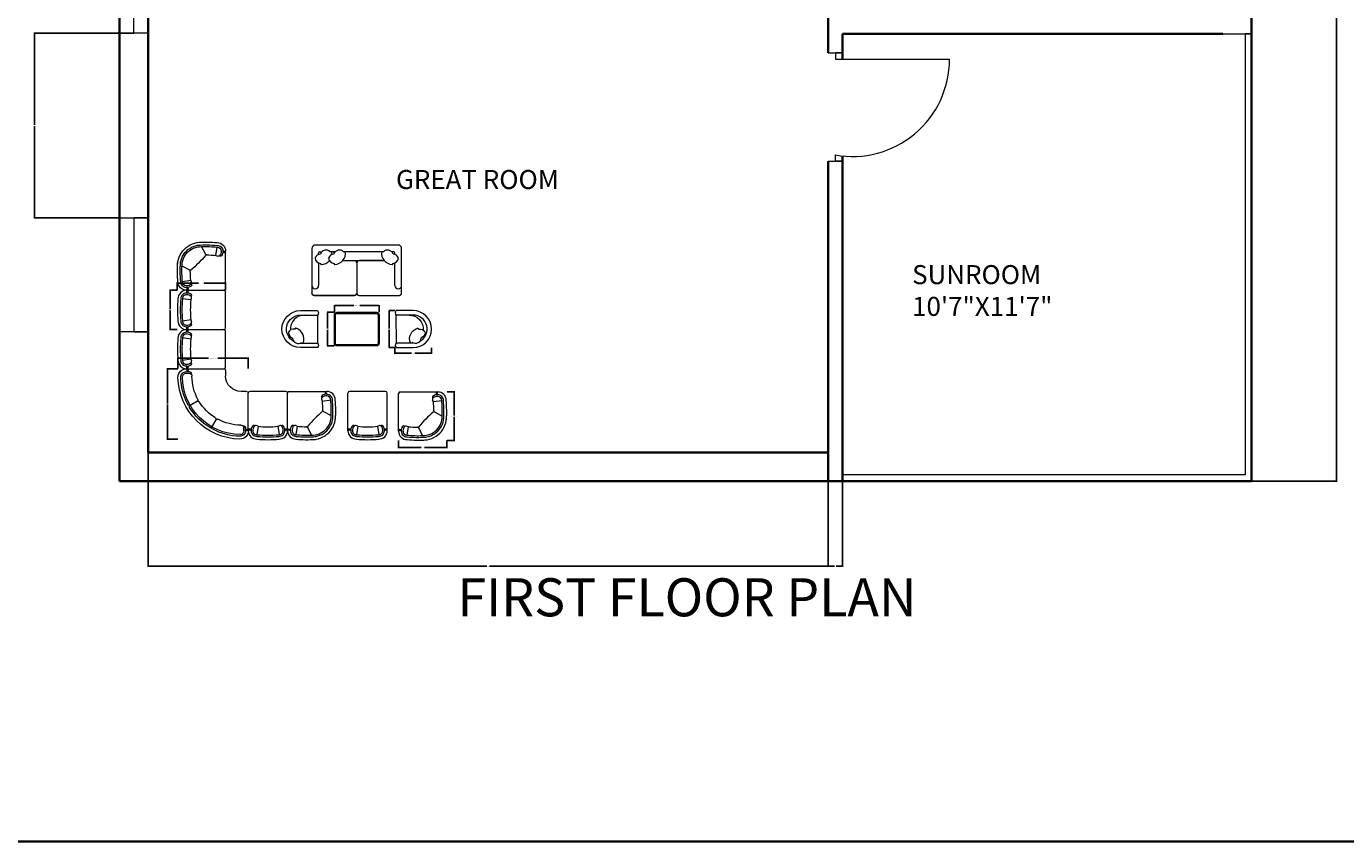
# Model space of a CAD drawing. Units: inches. Extents: x 1912 to 3731, y 1384 to 2459.
# Tile 3 of 8: x 2405 to 2821, y 1384 to 1641. Entities that reach past the tile are written whole.
import ezdxf

# ---------------------------------------------------------------- set-up
doc = ezdxf.new("R2010")
doc.units = ezdxf.units.IN
for name, color, linetype, lineweight in [('A-ANNO-DIMS', 2, 'Continuous', 18), ('A-ANNO-TITL', 7, 'Continuous', 25), ('A-ANNO-TTLB', 7, 'Continuous', 35), ('A-AREA-IDEN', 7, 'Continuous', 18), ('A-DOOR', 3, 'Continuous', 20), ('A-FURN', 8, 'Continuous', 15), ('A-GLAZ', 4, 'Continuous', 18), ('A-WALL', 7, 'Continuous', 35)]:
    doc.layers.add(name, color=color, linetype=linetype, lineweight=lineweight)
doc.styles.get("Standard").update_dxf_attribs({"font": 'arial.ttf'})
doc.dimstyles.get("Standard").update_dxf_attribs({"dimtxt": 0.18, "dimasz": 0.18, "dimexe": 0.18, "dimexo": 0.0625, "dimgap": 0.09, "dimtad": 0, "dimtih": 1, "dimtoh": 1, "dimdec": 4, "dimzin": 0, "dimdsep": 46, "dimtxsty": 'Standard', "dimcen": 0.09, "dimadec": 0, "dimazin": 0, "dimtfac": 1, "dimtdec": 4, "dimtofl": 0, "dimtmove": 0, "dimatfit": 3, "dimfxl": 1, "dimtolj": 1, "dimtzin": 0, "dimarcsym": 0})

# ---------------------------------------------------------------- blocks, each defined once
blk = doc.blocks.new('A$C707258B2')
at = {"color": 0}
for p, q in [((0.404, 0.342), (1.074, 0.342)), ((0.404, 0.292), (0.454, 0.292)), ((0.404, 0.262), (0.454, 0.262)), ((1.104, 0.312), (1.104, 0.212)), ((1.479, -0.063), (1.379, -0.063)), ((1.509, -0.763), (1.509, -0.093)), ((0.6, -0.238), (0.47, -0.313)), ((0.929, -0.567), (0.854, -0.697)), ((1.429, -0.763), (1.429, -0.713)), ((1.459, -0.763), (1.459, -0.712))]:
    blk.add_line(p, q, dxfattribs=at)
for centre, radius, start, end in [((0.404, 0.192), 0.15, 90, 181.1754), ((0.404, 0.192), 0.1, 90, 181.1754), ((0.404, 0.192), 0.07, 90, 181.1754), ((0.378, 0.317), 0.0362, 316.3972, 43.6028), ((0.368, 0.317), 0.0662, 337.8298, 22.1702), ((0.455, 0.256), 0.0357, 345.4262, 90.5555), ((0.454, 0.212), 0.05, 360, 90), ((1.074, 0.312), 0.03, 360, 90), ((1.379, 0.212), 1.125, 181.1754, 268.8246), ((1.379, 0.212), 1.075, 181.1754, 208.6357), ((1.379, 0.212), 1.045, 181.1754, 268.8246), ((1.379, 0.212), 0.875, 180, 208.4082), ((1.379, 0.212), 0.275, 180, 270), ((0.587, -0.216), 0.025, 300, 28.4082), ((0.612, -0.259), 0.025, 31.5918, 120), ((1.479, -0.093), 0.03, 360, 90), ((0.457, -0.291), 0.025, 208.6357, 300), ((0.482, -0.334), 0.025, 120, 211.3643), ((1.379, 0.212), 1.075, 211.3643, 238.6357), ((1.379, 0.212), 0.875, 211.5918, 238.4082), ((0.832, -0.685), 0.025, 238.6357, 330), ((0.876, -0.71), 0.025, 150, 241.3643), ((0.907, -0.555), 0.025, 330, 58.4082), ((0.951, -0.58), 0.025, 61.5918, 150), ((1.379, 0.212), 0.875, 241.5918, 270), ((1.379, -0.713), 0.05, 360, 90), ((1.425, -0.709), 0.0336, 354.6301, 109.3883), ((1.379, 0.212), 1.075, 241.3643, 268.8246), ((1.359, -0.763), 0.15, 268.8246, 360), ((1.359, -0.763), 0.1, 268.8246, 360), ((1.359, -0.763), 0.07, 268.8246, 360), ((1.484, -0.799), 0.0662, 67.8298, 112.1702), ((1.484, -0.789), 0.0362, 46.3972, 133.6028)]:
    blk.add_arc(centre, radius, start, end, dxfattribs=at)
blk = doc.blocks.new('A$C1352')
at = {"color": 0}
for points in [[(0.003, 0.053), (0.003, 0.553, -0.414214), (0.053, 0.603), (0.753, 0.603, -0.414214), (0.803, 0.553), (0.803, 0.053, -0.414214), (0.753, 0.003), (0.053, 0.003, -0.414214)], [(0.023, 0.053), (0.023, 0.553, -0.414214), (0.053, 0.583), (0.753, 0.583, -0.414214), (0.783, 0.553), (0.783, 0.053, -0.414214), (0.753, 0.023), (0.053, 0.023, -0.414214)]]:
    blk.add_lwpolyline(points, format="xyb", close=True, dxfattribs=at)
blk = doc.blocks.new('part 01')
at = {"color": 0}
for p, q in [((-591, 527), (-740, 550)), ((-670, 700), (0, 700)), ((-591, 527), (-579, 561)), ((30, 30), (30, 670)), ((-591, 173), (-740, 150)), ((-670, 0), (0, 0)), ((-591, 173), (-579, 139))]:
    blk.add_line(p, q, dxfattribs=at)
for centre, radius, start, end in [((1178, 350), 2008, 174.2835, 185.7165), ((-670, 550), 150, 90, 181.1754), ((1178, 350), 1958, 174.2835, 185.7165), ((-670, 550), 100, 90, 181.1754), ((1178, 350), 1928, 174.2835, 185.7165), ((-670, 550), 70, 90, 181.1754), ((-660, 518), 133, 56.0897, 95.6132), ((-696, 675), 36.2, 316.3972, 43.6028), ((-660, 518), 103, 42.0066, 95.6132), ((-706, 675), 66.2, 337.8298, 22.1702), ((1178, 350), 1778, 174.2835, 185.7165), ((-600, 607), 25, 332.9608, 56.0897), ((-625, 620), 53.2, 321.0017, 332.9608), ((-602, 570), 25, 340, 42.0066), ((0, 670), 30, 0, 90), ((-670, 150), 150, 178.8246, 270), ((-670, 150), 100, 178.8246, 270), ((-670, 150), 70, 178.8246, 270), ((-660, 182), 133, 264.3868, 303.9103), ((-660, 182), 103, 264.3868, 317.9934), ((-696, 25), 36.2, 316.3972, 43.6028), ((-706, 25), 66.2, 337.8298, 22.1702), ((-600, 93), 25, 303.9103, 27.0392), ((-602, 130), 25, 317.9934, 20), ((-625, 80), 53.2, 27.0392, 38.9983), ((0, 30), 30, 270, 0)]:
    blk.add_arc(centre, radius, start, end, dxfattribs=at)
blk = doc.blocks.new('part02')
at = {"color": 0}
for p, q in [((0, -670), (0, 0)), ((30, 30), (700, 30)), ((621, -143), (609, -109)), ((621, -143), (770, -120)), ((640, -326), (778, -399)), ((173, -591), (139, -579)), ((173, -591), (150, -740)), ((356, -610), (429, -748))]:
    blk.add_line(p, q, dxfattribs=at)
for centre, radius, start, end in [((30, 0), 30, 90, 180), ((726, 5), 56.2, 153.6122, 206.6666), ((726, 5), 36.2, 136.3972, 223.6028), ((700, -120), 150, 0, 90), ((630, -63), 25, 123.9103, 207.0392), ((655, -50), 53.2, 207.0392, 218.9983), ((632, -100), 25, 137.9934, 200), ((690, -152), 103, 84.3868, 137.9934), ((689, -151), 132, 85.4378, 123.9887), ((-1148, -320), 1778, 0.3836, 5.7165), ((700, -121), 101, 357.5006, 89.858), ((700, -120), 70, 0, 90), ((-1228, -320), 2008, 357.7349, 5.7032), ((-1148, -320), 1958, 355.8657, 5.7165), ((-1148, -320), 2008, 355.818, 5.7165), ((2220, -2190), 2454, 130.6961, 139.3039), ((439, -409), 419, 268.2181, 1.7819), ((439, -409), 369, 268.2181, 1.7819), ((439, -409), 339, 268.2181, 1.7819), ((632, -344), 20, 62, 130.6961), ((650, -308), 20, 180.3836, 242), ((25, -696), 56.2, 63.3334, 116.3878), ((25, -696), 36.2, 46.3972, 133.6028), ((150, -670), 150, 180, 271.1754), ((182, -660), 133, 146.0897, 185.6132), ((150, -670), 100, 180, 271.1754), ((93, -600), 25, 62.9608, 146.0897), ((182, -660), 103, 132.0066, 185.6132), ((150, -670), 70, 180, 270), ((80, -625), 53.2, 51.0017, 62.9608), ((130, -602), 25, 70, 132.0066), ((350, 1178), 1778, 264.2835, 269.6164), ((338, -620), 20, 28, 89.6164), ((374, -602), 20, 139.3039, 208), ((350, 1258), 2008, 264.2968, 272.2651), ((350, 1178), 2008, 264.2835, 274.182), ((350, 1178), 1958, 264.2835, 274.1343)]:
    blk.add_arc(centre, radius, start, end, dxfattribs=at)
blk = doc.blocks.new('LOUNGE-CHAIR')
blk.add_line((5.83, 1.42), (11.22, 1.41))
at = {"ltscale": 0.03}
blk.add_lwpolyline([(11.22, 1.41, -0.369229), (11.22, 0), (5.83, 0, -1), (5.84, 11.67), (11.23, 11.67, -0.369229), (11.23, 10.25)], format="xyb", close=True, dxfattribs=at)
blk.add_lwpolyline([(3.79, 1.92, -0.785087), (5.84, 10.26), (11.23, 10.25)], format="xyb")
for centre, radius, start, end in [((7.08, 5.84), 4.42, 89.9461, 183.658), ((3.71, 4.07), 1.82, 76.6403, 159.4695), ((4, 4.88), 1.99, 184.9999, 251.3534), ((4.33, 5.92), 0.211, 60.6238, 203.7423), ((3.5, 2.81), 3.42, 337.0143, 74.2857), ((5.13, 3.08), 1.77, 182.9922, 304.1401), ((5.83, 5.84), 4.42, 268.8536, 269.9461)]:
    blk.add_arc(centre, radius, start, end)
blk = doc.blocks.new('DOOR-36-FF-SUNROOM')
for p, q in [((0, 34.16), (4.5, 34.16)), ((4.5, 34.16), (2.25, 34.16)), ((2.25, 34.16), (2.25, 32.16)), ((2.25, 32.16), (38.25, 32.16)), ((2.25, 0), (2.25, 2)), ((0, 0), (4.5, 0)), ((4.5, 0), (2.25, 0))]:
    blk.add_line(p, q)
blk.add_arc((7.62, 32.16), 30.63, 259.9112, 0)
blk = doc.blocks.new('WIN-PLAN-60-B')
for p, q in [((0, 60), (9, 60)), ((9, 60), (4.5, 60)), ((4.5, 60), (4.5, 0)), ((9, 0), (0, 0)), ((4.5, 0), (9, 0))]:
    blk.add_line(p, q)
blk = doc.blocks.new('WIN-PLAN-36')
for p, q in [((4.5, 36), (0, 36)), ((0, 36), (9, 36)), ((4.5, 0), (4.5, 36)), ((9, 0), (0, 0)), ((0, 0), (4.5, 0))]:
    blk.add_line(p, q)
blk = doc.blocks.new('*D51')
at = {"layer": 'A-ANNO-DIMS', "color": 0, "lineweight": -2, "transparency": 16777216}
for p, q in [((2521.09, 1551.36), (2519.22, 1551.36)), ((2519.4, 1551.18), (2519.4, 1545.7)), ((2519.4, 1539.86), (2519.4, 1545.34)), ((2521.09, 1539.68), (2519.22, 1539.68))]:
    blk.add_line(p, q, dxfattribs=at)
at = {"layer": 'A-ANNO-DIMS', "color": 0, "transparency": 16777216}
for points in [[(2519.37, 1551.18), (2519.43, 1551.18), (2519.4, 1551.36)], [(2519.37, 1539.86), (2519.43, 1539.86), (2519.4, 1539.68)]]:
    blk.add_solid(points, dxfattribs=at)
at = {"layer": 'Defpoints', "color": 0, "transparency": 16777216}
for p in [(2519.4, 1551.36), (2521.15, 1551.36), (2521.15, 1539.68)]:
    blk.add_point(p, dxfattribs=at)
at = {"layer": 'A-ANNO-DIMS', "color": 0, "transparency": 16777216, "insert": (2519.4, 1545.52), "char_height": 0.18, "attachment_point": 5}
blk.add_mtext('\\A1;CHAIR 12 TYP.', dxfattribs=at)
blk = doc.blocks.new('*D52')
at = {"layer": 'A-ANNO-DIMS', "color": 0, "lineweight": -2, "transparency": 16777216}
for p, q in [((2521.15, 1539.62), (2521.15, 1537.75)), ((2532.73, 1539.62), (2532.73, 1537.75)), ((2521.33, 1537.93), (2526.42, 1537.93)), ((2532.55, 1537.93), (2527.46, 1537.93))]:
    blk.add_line(p, q, dxfattribs=at)
at = {"layer": 'A-ANNO-DIMS', "color": 0, "transparency": 16777216}
for points in [[(2521.33, 1537.96), (2521.33, 1537.9), (2521.15, 1537.93)], [(2532.55, 1537.96), (2532.55, 1537.9), (2532.73, 1537.93)]]:
    blk.add_solid(points, dxfattribs=at)
at = {"layer": 'Defpoints', "color": 0, "transparency": 16777216}
for p in [(2521.15, 1539.68), (2532.73, 1539.68), (2521.15, 1537.93)]:
    blk.add_point(p, dxfattribs=at)
at = {"layer": 'A-ANNO-DIMS', "color": 0, "transparency": 16777216, "insert": (2526.94, 1537.93), "char_height": 0.18, "attachment_point": 5}
blk.add_mtext('\\A1;12 TYP.', dxfattribs=at)
blk = doc.blocks.new('*D53')
at = {"layer": 'A-ANNO-DIMS', "color": 0, "lineweight": -2, "transparency": 16777216}
for p, q in [((2452.52, 1557.83), (2452.52, 1560.24)), ((2467.77, 1557.83), (2467.77, 1560.24)), ((2452.7, 1560.06), (2459.25, 1560.06)), ((2467.59, 1560.06), (2461.04, 1560.06))]:
    blk.add_line(p, q, dxfattribs=at)
at = {"layer": 'A-ANNO-DIMS', "color": 0, "transparency": 16777216}
for points in [[(2452.7, 1560.09), (2452.7, 1560.03), (2452.52, 1560.06)], [(2467.59, 1560.09), (2467.59, 1560.03), (2467.77, 1560.06)]]:
    blk.add_solid(points, dxfattribs=at)
at = {"layer": 'Defpoints', "color": 0, "transparency": 16777216}
for p in [(2452.52, 1557.77), (2467.77, 1560.06), (2467.77, 1557.77)]:
    blk.add_point(p, dxfattribs=at)
at = {"layer": 'A-ANNO-DIMS', "color": 0, "transparency": 16777216, "insert": (2460.15, 1560.06), "char_height": 0.18, "attachment_point": 5}
blk.add_mtext('\\A1;SEAT 15 TYP.', dxfattribs=at)
blk = doc.blocks.new('*D54')
at = {"layer": 'A-ANNO-DIMS', "color": 0, "lineweight": -2, "transparency": 16777216}
for p, q in [((2452.45, 1557.77), (2450.05, 1557.77)), ((2450.23, 1557.59), (2450.23, 1551.76)), ((2450.23, 1545.57), (2450.23, 1551.4)), ((2452.45, 1545.39), (2450.05, 1545.39))]:
    blk.add_line(p, q, dxfattribs=at)
at = {"layer": 'A-ANNO-DIMS', "color": 0, "transparency": 16777216}
for points in [[(2450.2, 1557.59), (2450.26, 1557.59), (2450.23, 1557.77)], [(2450.2, 1545.57), (2450.26, 1545.57), (2450.23, 1545.39)]]:
    blk.add_solid(points, dxfattribs=at)
at = {"layer": 'Defpoints', "color": 0, "transparency": 16777216}
for p in [(2450.23, 1557.77), (2452.52, 1557.77), (2452.52, 1545.39)]:
    blk.add_point(p, dxfattribs=at)
at = {"layer": 'A-ANNO-DIMS', "color": 0, "transparency": 16777216, "insert": (2450.23, 1551.58), "char_height": 0.18, "attachment_point": 5}
blk.add_mtext('\\A1;12 TYP.', dxfattribs=at)
blk = doc.blocks.new('*D55')
at = {"layer": 'A-ANNO-DIMS', "color": 0, "lineweight": -2, "transparency": 16777216}
for p, q in [((2537.62, 1525.71), (2540.02, 1525.71)), ((2539.84, 1525.53), (2539.84, 1518.27)), ((2539.84, 1510.64), (2539.84, 1517.91)), ((2537.62, 1510.46), (2540.02, 1510.46))]:
    blk.add_line(p, q, dxfattribs=at)
at = {"layer": 'A-ANNO-DIMS', "color": 0, "transparency": 16777216}
for points in [[(2539.81, 1525.53), (2539.87, 1525.53), (2539.84, 1525.71)], [(2539.81, 1510.64), (2539.87, 1510.64), (2539.84, 1510.46)]]:
    blk.add_solid(points, dxfattribs=at)
at = {"layer": 'Defpoints', "color": 0, "transparency": 16777216}
for p in [(2537.56, 1525.71), (2539.84, 1525.71), (2537.56, 1510.46)]:
    blk.add_point(p, dxfattribs=at)
at = {"layer": 'A-ANNO-DIMS', "color": 0, "transparency": 16777216, "insert": (2539.84, 1518.09), "char_height": 0.18, "attachment_point": 5}
blk.add_mtext('\\A1;END SEAT 15 TYP.', dxfattribs=at)
blk = doc.blocks.new('*D56')
at = {"layer": 'A-ANNO-DIMS', "color": 0, "lineweight": -2, "transparency": 16777216}
for p, q in [((2522.3, 1510.4), (2522.3, 1508)), ((2537.56, 1510.4), (2537.56, 1508)), ((2522.48, 1508.18), (2529.41, 1508.18)), ((2537.38, 1508.18), (2530.45, 1508.18))]:
    blk.add_line(p, q, dxfattribs=at)
at = {"layer": 'A-ANNO-DIMS', "color": 0, "transparency": 16777216}
for points in [[(2522.48, 1508.21), (2522.48, 1508.15), (2522.3, 1508.18)], [(2537.38, 1508.21), (2537.38, 1508.15), (2537.56, 1508.18)]]:
    blk.add_solid(points, dxfattribs=at)
at = {"layer": 'Defpoints', "color": 0, "transparency": 16777216}
for p in [(2522.3, 1510.46), (2537.56, 1510.46), (2537.56, 1508.18)]:
    blk.add_point(p, dxfattribs=at)
at = {"layer": 'A-ANNO-DIMS', "color": 0, "transparency": 16777216, "insert": (2529.93, 1508.18), "char_height": 0.18, "attachment_point": 5}
blk.add_mtext('\\A1;15 TYP.', dxfattribs=at)
blk = doc.blocks.new('*D57')
at = {"layer": 'A-ANNO-DIMS', "color": 0, "lineweight": -2, "transparency": 16777216}
for p, q in [((2452.74, 1533.08), (2452.74, 1536.53)), ((2452.92, 1536.35), (2462.36, 1536.35)), ((2474.75, 1536.35), (2465.31, 1536.35)), ((2474.93, 1533.08), (2474.93, 1536.53))]:
    blk.add_line(p, q, dxfattribs=at)
at = {"layer": 'A-ANNO-DIMS', "color": 0, "transparency": 16777216}
for points in [[(2452.92, 1536.38), (2452.92, 1536.32), (2452.74, 1536.35)], [(2474.75, 1536.38), (2474.75, 1536.32), (2474.93, 1536.35)]]:
    blk.add_solid(points, dxfattribs=at)
at = {"layer": 'Defpoints', "color": 0, "transparency": 16777216}
for p in [(2474.93, 1536.35), (2452.74, 1533.02), (2474.93, 1533.02)]:
    blk.add_point(p, dxfattribs=at)
at = {"layer": 'A-ANNO-DIMS', "color": 0, "transparency": 16777216, "insert": (2463.83, 1536.35), "char_height": 0.18, "attachment_point": 5}
blk.add_mtext('\\A1;CORNER SEAT 22 TYP.', dxfattribs=at)
blk = doc.blocks.new('*D58')
at = {"layer": 'A-ANNO-DIMS', "color": 0, "lineweight": -2, "transparency": 16777216}
for p, q in [((2452.68, 1533.02), (2449.23, 1533.02)), ((2449.41, 1532.84), (2449.41, 1522.11)), ((2449.41, 1511.01), (2449.41, 1521.74)), ((2452.68, 1510.83), (2449.23, 1510.83))]:
    blk.add_line(p, q, dxfattribs=at)
at = {"layer": 'A-ANNO-DIMS', "color": 0, "transparency": 16777216}
for points in [[(2449.38, 1532.84), (2449.44, 1532.84), (2449.41, 1533.02)], [(2449.38, 1511.01), (2449.44, 1511.01), (2449.41, 1510.83)]]:
    blk.add_solid(points, dxfattribs=at)
at = {"layer": 'Defpoints', "color": 0, "transparency": 16777216}
for p in [(2449.41, 1533.02), (2452.74, 1533.02), (2452.74, 1510.83)]:
    blk.add_point(p, dxfattribs=at)
at = {"layer": 'A-ANNO-DIMS', "color": 0, "transparency": 16777216, "insert": (2449.41, 1521.92), "char_height": 0.18, "attachment_point": 5}
blk.add_mtext('\\A1;22 TYP.', dxfattribs=at)
blk = doc.blocks.new('*D59')
at = {"layer": 'A-ANNO-DIMS', "color": 0, "lineweight": -2, "transparency": 16777216}
for p, q in [((2502.06, 1550.88), (2502.06, 1553.12)), ((2502.24, 1552.94), (2508.17, 1552.94)), ((2516.02, 1552.94), (2510.1, 1552.94)), ((2516.2, 1550.88), (2516.2, 1553.12))]:
    blk.add_line(p, q, dxfattribs=at)
at = {"layer": 'A-ANNO-DIMS', "color": 0, "transparency": 16777216}
for points in [[(2502.24, 1552.97), (2502.24, 1552.91), (2502.06, 1552.94)], [(2516.02, 1552.97), (2516.02, 1552.91), (2516.2, 1552.94)]]:
    blk.add_solid(points, dxfattribs=at)
at = {"layer": 'Defpoints', "color": 0, "transparency": 16777216}
for p in [(2516.2, 1552.94), (2502.06, 1550.82), (2516.2, 1550.82)]:
    blk.add_point(p, dxfattribs=at)
at = {"layer": 'A-ANNO-DIMS', "color": 0, "transparency": 16777216, "insert": (2509.13, 1552.94), "char_height": 0.18, "attachment_point": 5}
blk.add_mtext('\\A1;TABLE 14 TYP.', dxfattribs=at)
blk = doc.blocks.new('*D60')
at = {"layer": 'A-ANNO-DIMS', "color": 0, "lineweight": -2, "transparency": 16777216}
for p, q in [((2502, 1550.82), (2499.76, 1550.82)), ((2499.94, 1550.64), (2499.94, 1545.7)), ((2499.94, 1540.39), (2499.94, 1545.34)), ((2502, 1540.21), (2499.76, 1540.21))]:
    blk.add_line(p, q, dxfattribs=at)
at = {"layer": 'A-ANNO-DIMS', "color": 0, "transparency": 16777216}
for points in [[(2499.91, 1550.64), (2499.97, 1550.64), (2499.94, 1550.82)], [(2499.91, 1540.39), (2499.97, 1540.39), (2499.94, 1540.21)]]:
    blk.add_solid(points, dxfattribs=at)
at = {"layer": 'Defpoints', "color": 0, "transparency": 16777216}
for p in [(2499.94, 1550.82), (2502.06, 1550.82), (2502.06, 1540.21)]:
    blk.add_point(p, dxfattribs=at)
at = {"layer": 'A-ANNO-DIMS', "color": 0, "transparency": 16777216, "insert": (2499.94, 1545.52), "char_height": 0.18, "attachment_point": 5}
blk.add_mtext('\\A1;11 TYP.', dxfattribs=at)
blk = doc.blocks.new('*D100')
at = {"layer": 'A-ANNO-DIMS', "color": 0, "lineweight": -2, "transparency": 16777216}
for p, q in [((2791.37, 1973.13), (2818.34, 1973.13)), ((2818.16, 1972.95), (2818.16, 1735.56)), ((2818.16, 1497.81), (2818.16, 1735.19)), ((2791.37, 1497.63), (2818.34, 1497.63))]:
    blk.add_line(p, q, dxfattribs=at)
at = {"layer": 'A-ANNO-DIMS', "color": 0, "transparency": 16777216}
for points in [[(2818.13, 1972.95), (2818.19, 1972.95), (2818.16, 1973.13)], [(2818.13, 1497.81), (2818.19, 1497.81), (2818.16, 1497.63)]]:
    blk.add_solid(points, dxfattribs=at)
at = {"layer": 'Defpoints', "color": 0, "transparency": 16777216}
for p in [(2791.31, 1973.13), (2818.16, 1973.13), (2791.31, 1497.63)]:
    blk.add_point(p, dxfattribs=at)
at = {"layer": 'A-ANNO-DIMS', "color": 0, "transparency": 16777216, "insert": (2818.16, 1735.38), "char_height": 0.18, "attachment_point": 5}
blk.add_mtext('\\A1;475.5', dxfattribs=at)
blk = doc.blocks.new('*D102')
at = {"layer": 'A-ANNO-DIMS', "color": 0, "lineweight": -2, "transparency": 16777216}
for p, q in [((2434.25, 1638.78), (2407.28, 1638.78)), ((2407.46, 1638.6), (2407.46, 1609.89)), ((2407.46, 1580.82), (2407.46, 1609.53)), ((2434.25, 1580.64), (2407.28, 1580.64))]:
    blk.add_line(p, q, dxfattribs=at)
at = {"layer": 'A-ANNO-DIMS', "color": 0, "transparency": 16777216}
for points in [[(2407.43, 1638.6), (2407.49, 1638.6), (2407.46, 1638.78)], [(2407.43, 1580.82), (2407.49, 1580.82), (2407.46, 1580.64)]]:
    blk.add_solid(points, dxfattribs=at)
at = {"layer": 'Defpoints', "color": 0, "transparency": 16777216}
for p in [(2407.46, 1638.78), (2434.31, 1638.78), (2434.31, 1580.64)]:
    blk.add_point(p, dxfattribs=at)
at = {"layer": 'A-ANNO-DIMS', "color": 0, "transparency": 16777216, "insert": (2407.46, 1609.71), "char_height": 0.18, "attachment_point": 5}
blk.add_mtext('\\A1;58.15', dxfattribs=at)
blk = doc.blocks.new('*D103')
at = {"layer": 'A-ANNO-DIMS', "color": 0, "lineweight": -2, "transparency": 16777216}
for p, q in [((2443.31, 1506.56), (2443.31, 1470.6)), ((2657.81, 1506.56), (2657.81, 1470.6)), ((2443.49, 1470.78), (2550.17, 1470.78)), ((2657.63, 1470.78), (2550.96, 1470.78))]:
    blk.add_line(p, q, dxfattribs=at)
at = {"layer": 'A-ANNO-DIMS', "color": 0, "transparency": 16777216}
for points in [[(2443.49, 1470.81), (2443.49, 1470.75), (2443.31, 1470.78)], [(2657.63, 1470.81), (2657.63, 1470.75), (2657.81, 1470.78)]]:
    blk.add_solid(points, dxfattribs=at)
at = {"layer": 'Defpoints', "color": 0, "transparency": 16777216}
for p in [(2443.31, 1506.63), (2657.81, 1506.63), (2657.81, 1470.78)]:
    blk.add_point(p, dxfattribs=at)
at = {"layer": 'A-ANNO-DIMS', "color": 0, "transparency": 16777216, "insert": (2550.56, 1470.78), "char_height": 0.18, "attachment_point": 5}
blk.add_mtext('\\A1;214.5', dxfattribs=at)
blk = doc.blocks.new('*D104')
at = {"layer": 'A-ANNO-DIMS', "color": 0, "lineweight": -2, "transparency": 16777216}
for p, q in [((2657.81, 1497.56), (2657.81, 1470.6)), ((2662.31, 1497.56), (2662.31, 1470.6)), ((2657.99, 1470.78), (2659.8, 1470.78)), ((2662.13, 1470.78), (2660.32, 1470.78))]:
    blk.add_line(p, q, dxfattribs=at)
at = {"layer": 'A-ANNO-DIMS', "color": 0, "transparency": 16777216}
for points in [[(2657.99, 1470.81), (2657.99, 1470.75), (2657.81, 1470.78)], [(2662.13, 1470.81), (2662.13, 1470.75), (2662.31, 1470.78)]]:
    blk.add_solid(points, dxfattribs=at)
at = {"layer": 'Defpoints', "color": 0, "transparency": 16777216}
for p in [(2657.81, 1497.63), (2662.31, 1497.63), (2662.31, 1470.78)]:
    blk.add_point(p, dxfattribs=at)
at = {"layer": 'A-ANNO-DIMS', "color": 0, "transparency": 16777216, "insert": (2660.06, 1470.78), "char_height": 0.18, "attachment_point": 5}
blk.add_mtext('\\A1;4.5', dxfattribs=at)

msp = doc.modelspace()

# ---------------------------------------------------------------- linework, layer by layer
at = {"layer": 'A-ANNO-TTLB'}
msp.add_lwpolyline([(1912.2029, 2458.5537), (3720.218, 2458.5537), (3720.218, 1383.9599), (1912.2029, 1383.9599)], close=True, dxfattribs=at)
at = {"layer": 'A-FURN'}
for p, q in [((2497.1144, 1569.0629), (2497.1144, 1569.5551)), ((2497.4679, 1569.9086), (2498.1182, 1569.9086)), ((2502.3619, 1569.9086), (2500.6702, 1569.9086)), ((2501.7116, 1569.9086), (2502.3619, 1569.9086)), ((2517.597, 1569.9086), (2504.9139, 1569.9086)), ((2520.7994, 1569.9086), (2520.149, 1569.9086)), ((2521.1529, 1569.0629), (2521.1529, 1569.5551)), ((2497.1144, 1566.3798), (2497.1144, 1559.3034)), ((2521.1529, 1559.3034), (2521.1529, 1566.3798))]:
    msp.add_line(p, q, dxfattribs=at)
at = {"layer": 'A-FURN', "ltscale": 0.03}
msp.add_lwpolyline([(2509.1423, 1556.8289, 0.41421356), (2509.8493, 1556.1218), (2522.5669, 1556.1218, 0.41421356), (2523.2739, 1556.8289), (2523.2739, 1570.9691, 0.41421356), (2522.2134, 1572.0297), (2496.0539, 1572.0297, 0.41421356), (2494.9933, 1570.9691), (2494.9933, 1556.8289, 0.41421356), (2495.7004, 1556.1218), (2508.4179, 1556.1218, 0.41421356), (2509.1249, 1556.8289)], format="xyb", dxfattribs=at)
at = {"layer": 'A-FURN'}
for points in [[(2504.7721, 1567.1689), (2508.2499, 1567.1689, -0.41421356), (2509.1336, 1566.2852), (2509.1336, 1557.0056, -0.41421356), (2508.2499, 1556.1218), (2495.8771, 1556.1218, -0.41421356), (2494.9933, 1557.0056)], [(2517.1369, 1567.1689), (2510.0174, 1567.1689, 0.41421356), (2509.1336, 1566.2852), (2509.1336, 1557.0056, 0.41421356), (2510.0174, 1556.1218), (2522.3901, 1556.1218, 0.41421356), (2523.2739, 1557.0056)]]:
    msp.add_lwpolyline(points, format="xyb", dxfattribs=at)
msp.add_lwpolyline([(2504.7721, 1567.1689), (2517.7389, 1567.1689)], dxfattribs=at)
for centre, radius, start, end in [((2497.8594, 1567.2139), 1.9935, 94.543938, 160.89739), ((2497.4679, 1569.5551), 0.3535, 90, 180), ((2497.4679, 1569.5551), 0.3535, 90, 180), ((2499.3942, 1568.6805), 1.771, 41.757236, 162.905096), ((2502.1031, 1567.2139), 1.9935, 94.543938, 160.89739), ((2497.8836, 1569.3401), 3.4218, 354.880983, 8.88305), ((2503.6379, 1568.6805), 1.771, 41.757236, 162.905096), ((2502.1272, 1569.3401), 3.4218, 271.611631, 8.88305), ((2520.3837, 1569.3401), 3.4218, 171.11695, 268.388369), ((2518.873, 1568.6805), 1.771, 17.094904, 138.242764), ((2520.4079, 1567.2139), 1.9935, 19.10261, 85.456062), ((2520.7994, 1569.5551), 0.3535, 0, 90), ((2497.7807, 1568.0696), 1.8164, 186.427858, 269.256998), ((2497.9241, 1566.1236), 0.2114, 142.154994, 285.27353), ((2497.8836, 1569.3401), 3.4218, 271.611631, 319.375991), ((2502.0244, 1568.0696), 1.8164, 186.427858, 269.256998), ((2502.1678, 1566.1236), 0.2114, 142.154994, 285.27353), ((2520.3431, 1566.1236), 0.2114, 254.72647, 37.845006), ((2520.4866, 1568.0696), 1.8164, 270.743002, 353.572142), ((2496.0539, 1559.3034), 1.0605, 180, 270), ((2496.0539, 1559.3034), 1.0605, 270, 0), ((2522.2134, 1559.3034), 1.0605, 180, 270), ((2522.2134, 1559.3034), 1.0605, 270, 0)]:
    msp.add_arc(centre, radius, start, end, dxfattribs=at)
at = {"layer": 'A-GLAZ'}
for p, q in [((2782.311, 1638.6258), (2791.311, 1638.6258)), ((2791.311, 1638.6258), (2789.311, 1638.6258)), ((2789.311, 1638.6258), (2789.311, 1499.6258)), ((2789.311, 1499.6258), (2662.311, 1499.6258))]:
    msp.add_line(p, q, dxfattribs=at)
at = {"layer": 'A-WALL'}
for p, q in [((2434.311, 1973.1258), (2434.311, 1497.6258)), ((2791.311, 1973.1258), (2791.311, 1497.6258)), ((2443.311, 1839.6258), (2443.311, 1506.6258)), ((2657.811, 1638.6258), (2657.811, 1726.8699)), ((2657.811, 1638.6258), (2657.811, 1632.5769)), ((2686.311, 1638.6258), (2662.311, 1638.6258)), ((2662.311, 1630.5769), (2662.311, 1638.6258)), ((2782.311, 1638.6258), (2686.311, 1638.6258)), ((2657.811, 1598.4168), (2657.811, 1497.6258)), ((2662.311, 1497.6258), (2662.311, 1600.1021)), ((2443.311, 1506.6258), (2657.811, 1506.6258)), ((2434.311, 1497.6258), (2791.311, 1497.6258)), ((2657.811, 1497.6258), (2662.311, 1497.6258))]:
    msp.add_line(p, q, dxfattribs=at)

# ---------------------------------------------------------------- block references
at = {"layer": 'A-DOOR'}
msp.add_blockref('DOOR-36-FF-SUNROOM', (2657.811, 1598.417), dxfattribs=at)
at = {"layer": 'A-FURN', "ltscale": 0.03}
for name, p, xscale, yscale, zscale, rotation in [('part02', (2467.2427, 1557.7668), -0.0176753547193075, 0.0176753547193075, 0.0176753547193075, 269.9999999999968), ('A$C707258B2', (2468.8861, 1506.3501), -17.67535471930751, 17.67535471930751, 17.67535471930751, 269.9999999999968), ('part 01', (2487.3042, 1525.3325), 0.0176753547193075, 0.0176753547193075, 0.0176753547193075, 90), ('part 01', (2518.7369, 1525.3325), 0.0176753547193075, 0.0176753547193075, 0.0176753547193075, 90)]:
    msp.add_blockref(name, p, dxfattribs=dict(at, xscale=xscale, yscale=yscale, zscale=zscale, rotation=rotation))
for name, p, xscale, yscale, zscale in [('part 01', (2467.2427, 1545.394), 0.0176753547193075, 0.0176753547193075, 0.0176753547193075), ('A$C1352', (2502.016, 1540.1611), 17.67535471930751, 17.67535471930751, 17.67535471930751), ('part 01', (2467.2427, 1533.0213), 0.0176753547193075, 0.0176753547193075, 0.0176753547193075), ('part02', (2487.3042, 1525.3325), 0.0176753547193075, 0.0176753547193075, 0.0176753547193075), ('part02', (2522.3038, 1525.1843), 0.0176753547193075, 0.0176753547193075, 0.0176753547193075)]:
    msp.add_blockref(name, p, dxfattribs=dict(at, xscale=xscale, yscale=yscale, zscale=zscale))
at = {"layer": 'A-FURN'}
msp.add_blockref('LOUNGE-CHAIR', (2485.5355, 1539.6842), dxfattribs=at)
at = {"layer": 'A-FURN', "extrusion": (0, 0, -1), "zscale": -1}
msp.add_blockref('LOUNGE-CHAIR', (-2532.7317, 1539.6842), dxfattribs=at)
at = {"layer": 'A-GLAZ', "rotation": 180}
for name, p in [('WIN-PLAN-60-B', (2443.3108, 1698.7837)), ('WIN-PLAN-36', (2443.3108, 1580.6377))]:
    msp.add_blockref(name, p, dxfattribs=at)

# ---------------------------------------------------------------- texts
at = {"layer": 'A-ANNO-TITL', "insert": (2540.8592, 1466.9787), "char_height": 12, "attachment_point": 1}
msp.add_mtext_dynamic_manual_height_columns('FIRST FLOOR PLAN', width=293.671814, gutter_width=12.5, heights=[0], dxfattribs=at)
at = {"layer": 'A-AREA-IDEN', "char_height": 6, "attachment_point": 1}
for s, width, insert in [('GREAT ROOM', 172.727967, (2521.5005, 1595.691)), ('SUNROOM\\P10\'7"X11\'7"', 147.862137, (2684.2725, 1565.6982))]:
    msp.add_mtext_dynamic_manual_height_columns(s, width=width, gutter_width=12.5, heights=[0], dxfattribs=dict(at, insert=insert))

# ---------------------------------------------------------------- dimensions: what is measured, and where the dimension line sits
at = {"layer": 'A-ANNO-DIMS'}
for base, p1, p2, override, picture, middle in [((2818.161, 1973.1258), (2791.311, 1497.6258), (2791.311, 1973.1258), {"dimdec": 1, "dimlfac": 1, "dimrnd": 0, "dimzin": 0, "dimdsep": 46, "dimlunit": 2}, '*D100', (2818.161, 1735.3758)), ((2407.461, 1638.7838), (2434.311, 1580.6379), (2434.311, 1638.7838), {"dimdec": 2, "dimlfac": 1, "dimrnd": 0, "dimzin": 0, "dimdsep": 46, "dimlunit": 2}, '*D102', (2407.461, 1609.7109))]:
    dim = msp.add_linear_dim(base=base, p1=p1, p2=p2, angle=90, dimstyle='Standard', override=override, dxfattribs=at)
    dim.commit()
    dim.dimension.update_dxf_attribs({"geometry": picture, "text_midpoint": middle})
for base, p1, p2, text, picture, middle in [((2467.7729, 1560.0551), (2452.5172, 1557.7668), (2467.7729, 1557.7668), 'SEAT <> TYP.', '*D53', (2460.145, 1560.0551)), ((2516.2038, 1552.9403), (2502.0635, 1550.8192), (2516.2038, 1550.8192), 'TABLE <> TYP.', '*D59', (2509.1336, 1552.9403)), ((2474.9314, 1536.3502), (2452.7384, 1533.0213), (2474.9314, 1533.0213), 'CORNER SEAT <> TYP.', '*D57', (2463.8349, 1536.3502)), ((2537.5554, 1508.1753), (2522.3038, 1510.463), (2537.5554, 1510.463), '<> TYP.', '*D56', (2529.9296, 1508.1753))]:
    dim = msp.add_linear_dim(base=base, p1=p1, p2=p2, text=text, dimstyle='Standard', override={"dimdec": 0, "dimlfac": 1, "dimrnd": 0, "dimzin": 0, "dimdsep": 46, "dimlunit": 2}, dxfattribs=at)
    dim.commit()
    dim.dimension.update_dxf_attribs({"geometry": picture, "text_midpoint": middle})
for base, p1, p2, angle, text, picture, middle in [((2450.2288, 1557.7668), (2452.5172, 1545.394), (2452.5172, 1557.7668), 90, '<> TYP.', '*D54', (2450.2288, 1551.5804)), ((2499.9424, 1550.8192), (2502.0635, 1540.214), (2502.0635, 1550.8192), 90, '<> TYP.', '*D60', (2499.9424, 1545.5166)), ((2519.4021, 1551.3576), (2521.1532, 1539.6838), (2521.1532, 1551.3576), 90, 'CHAIR <> TYP.', '*D51', (2519.4021, 1545.5207)), ((2521.1532, 1537.9327), (2532.7347, 1539.6838), (2521.1532, 1539.6838), 180, '<> TYP.', '*D52', (2526.944, 1537.9327)), ((2449.4095, 1533.0213), (2452.7384, 1510.8283), (2452.7384, 1533.0213), 90, '<> TYP.', '*D58', (2449.4095, 1521.9248)), ((2539.8431, 1525.7146), (2537.5554, 1510.463), (2537.5554, 1525.7146), 90, 'END SEAT <> TYP.', '*D55', (2539.8431, 1518.0888))]:
    dim = msp.add_linear_dim(base=base, p1=p1, p2=p2, angle=angle, text=text, dimstyle='Standard', override={"dimdec": 0, "dimlfac": 1, "dimrnd": 0, "dimzin": 0, "dimdsep": 46, "dimlunit": 2}, dxfattribs=at)
    dim.commit()
    dim.dimension.update_dxf_attribs({"geometry": picture, "text_midpoint": middle})
for base, p1, p2, picture, middle in [((2657.811, 1470.7758), (2443.311, 1506.6258), (2657.811, 1506.6258), '*D103', (2550.561, 1470.7758)), ((2662.311, 1470.7758), (2657.811, 1497.6258), (2662.311, 1497.6258), '*D104', (2660.061, 1470.7758))]:
    dim = msp.add_linear_dim(base=base, p1=p1, p2=p2, dimstyle='Standard', override={"dimdec": 1, "dimlfac": 1, "dimrnd": 0, "dimzin": 0, "dimdsep": 46, "dimlunit": 2}, dxfattribs=at)
    dim.commit()
    dim.dimension.update_dxf_attribs({"geometry": picture, "text_midpoint": middle})

doc.saveas('drawing.dxf')
